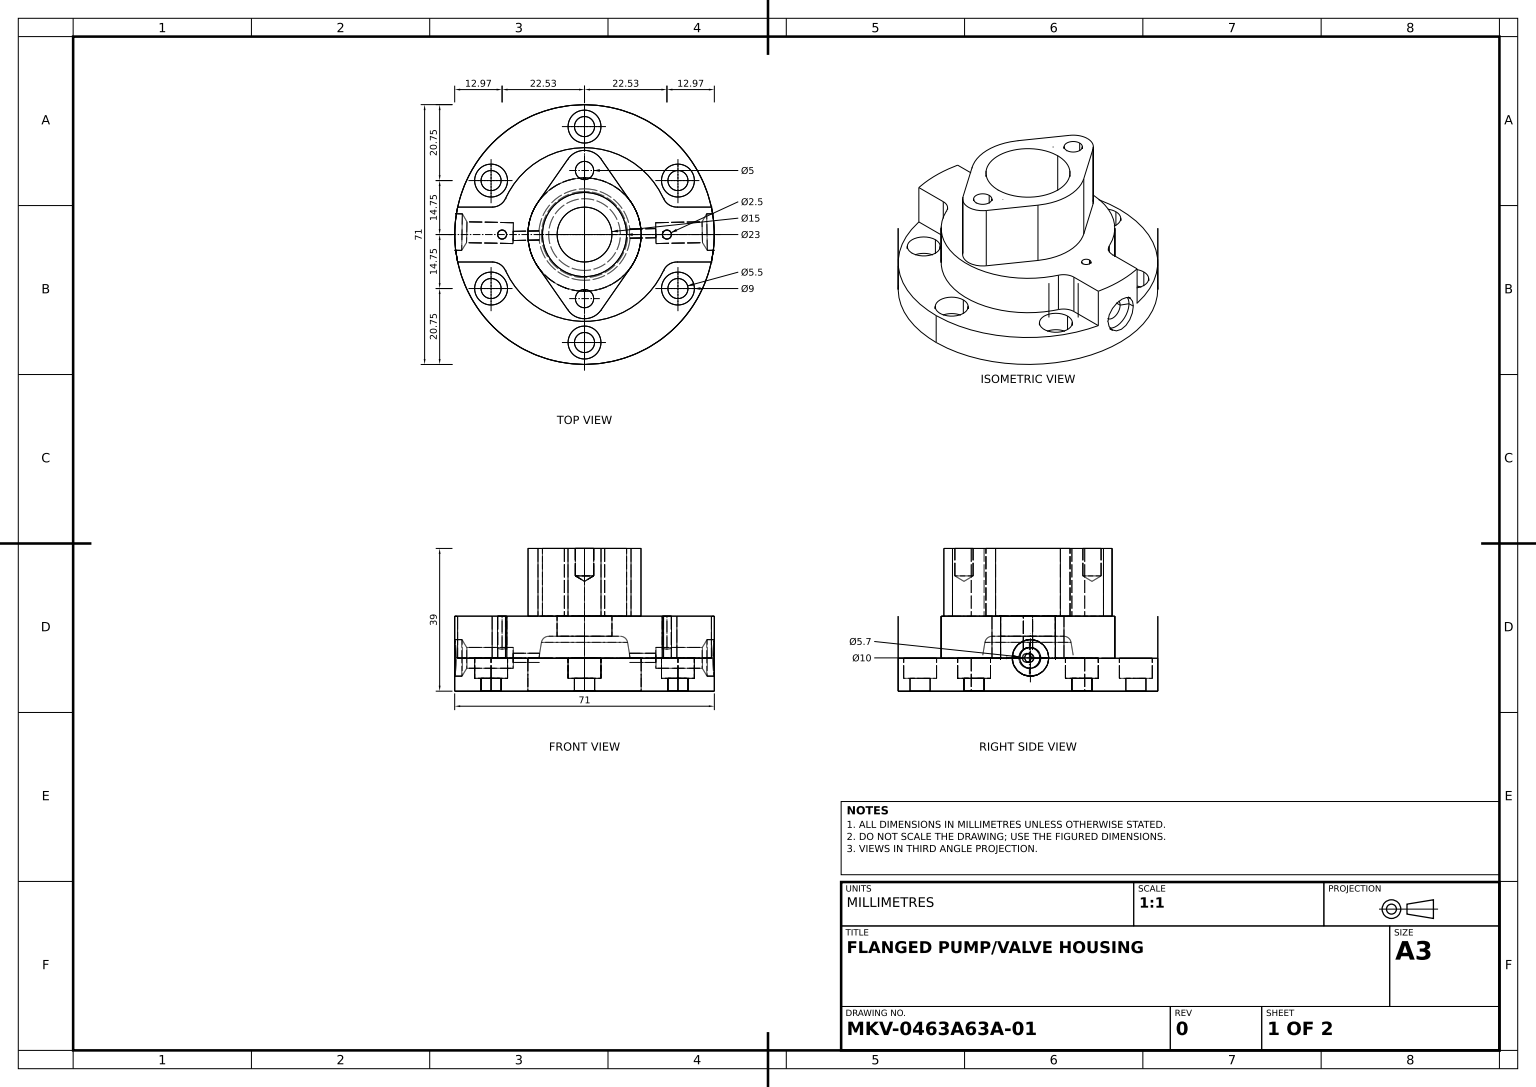
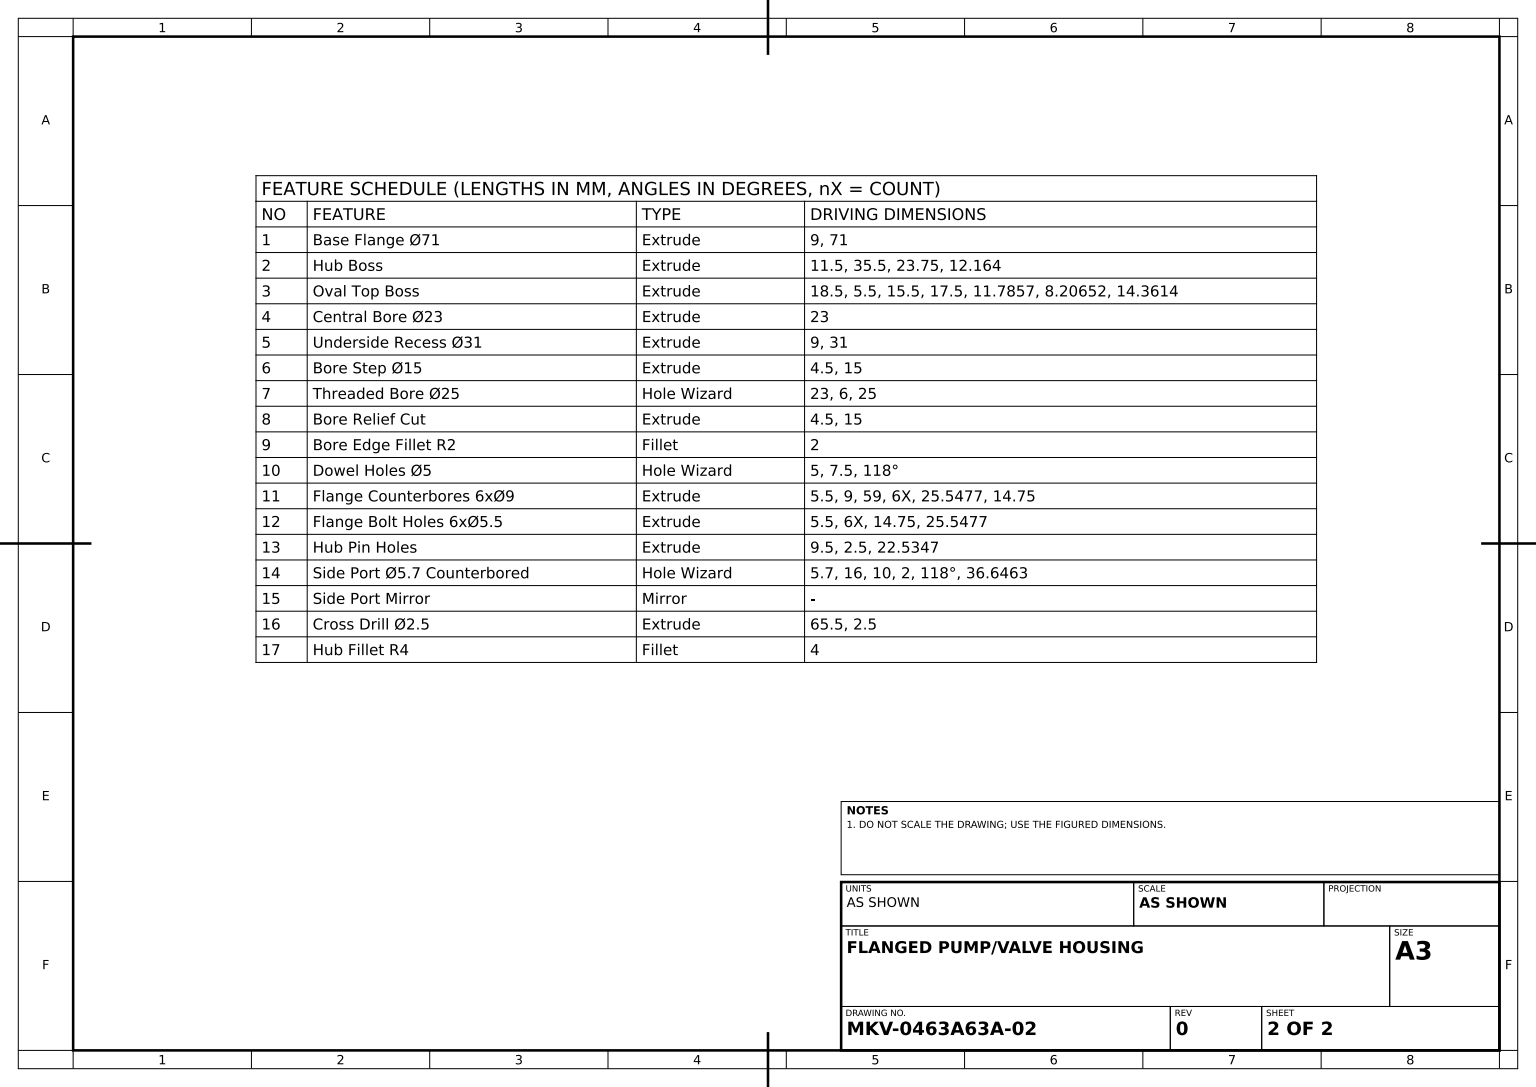
from build123d import *

# Parameters (mm, degrees)
BASE_FLANGE_SKETCH_R           = 35.5
BASE_FLANGE_71_DEPTH           = 9
HUB_BOSS_DEPTH                 = 11.5
OVAL_TOP_BOSS_DEPTH            = 18.5
CENTRAL_BORE_SKETCH_R          = 11.5
CENTRAL_BORE_23_DEPTH          = 18.5
UNDERSIDE_RECESS_SKETCH_R      = 15.5
UNDERSIDE_RECESS_31_DEPTH      = 9
BORE_STEP_SKETCH_R             = 7.5
BORE_STEP_15_DEPTH             = 4.5
BORE_RELIEF_SKETCH_R           = 7.5
BORE_RELIEF_CUT_DEPTH          = 4.5
BORE_EDGE_FILLET_R2_R          = 2
DOWEL_HOLES_5_D                = 5
DOWEL_HOLES_5_DEPTH            = 7.5
DOWEL_HOLES_5_TIP              = 1.502151548
FLANGE_COUNTERBORE_SKETCH_R    = 4.5
FLANGE_COUNTERBORES_6X_9_DEPTH = 5.5
FLANGE_BOLT_HOLE_SKETCH_R      = 2.75
FLANGE_BOLT_HOLES_6X_5_5_DEPTH = 5.5
HUB_PIN_HOLES_SKETCH_R         = 1.25
HUB_PIN_HOLES_DEPTH            = 9.5
CROSS_DRILL_SKETCH_R           = 1.25
CROSS_DRILL_2_5_DEPTH          = 65.5
HUB_FILLET_R4_R                = 4


with BuildPart() as part:
    # Base Flange Sketch → Base Flange _71 (new body)
    with BuildSketch(Plane(origin=(0, 0, 0), x_dir=(1, 0, 0), z_dir=(0, 1, 0))):
        with Locations(Location((0, 0, 0), (0, 0, 270))):
            Circle(BASE_FLANGE_SKETCH_R)
    extrude(amount=BASE_FLANGE_71_DEPTH)

    # Hub Profile Sketch → Hub Boss (add)
    with BuildSketch(Plane(origin=(0, 9, 0), x_dir=(1, 0, 0), z_dir=(0, 1, 0))):
        with BuildLine():
            Line((-22.534695472, 7.5), (-34.698703146, 7.5))
            ThreePointArc((-34.698703146, 7.5), (-35.5, 0), (-34.698703146, -7.5))
            Line((-34.698703146, -7.5), (-22.534695472, -7.5))
            ThreePointArc((-22.534695472, -7.5), (0, -23.75), (22.534695472, -7.5))
            Line((22.534695472, -7.5), (34.698703146, -7.5))
            ThreePointArc((34.698703146, -7.5), (35.5, 0), (34.698703146, 7.5))
            Line((34.698703146, 7.5), (22.534695472, 7.5))
            ThreePointArc((22.534695472, 7.5), (0, 23.75), (-22.534695472, 7.5))
        make_face()
    extrude(amount=HUB_BOSS_DEPTH)

    # Oval Top Boss Sketch → Oval Top Boss (add)
    with BuildSketch(Plane(origin=(0, 20.5, 0), x_dir=(1, 0, 0), z_dir=(0, 1, 0))):
        with BuildLine():
            Line((-4.513584937, 20.642857143), (-12.720103003, 8.857142857))
            ThreePointArc((-12.720103003, 8.857142857), (-15.5, 0), (-12.720103003, -8.857142857))
            Line((-12.720103003, -8.857142857), (-4.513584937, -20.642857143))
            ThreePointArc((-4.513584937, -20.642857143), (0, -23), (4.513584937, -20.642857143))
            Line((4.513584937, -20.642857143), (12.720103003, -8.857142857))
            ThreePointArc((12.720103003, -8.857142857), (15.5, 0), (12.720103003, 8.857142857))
            Line((12.720103003, 8.857142857), (4.513584937, 20.642857143))
            ThreePointArc((4.513584937, 20.642857143), (0, 23), (-4.513584937, 20.642857143))
        make_face()
    extrude(amount=OVAL_TOP_BOSS_DEPTH)

    # Central Bore Sketch → Central Bore _23 (cut)
    with BuildSketch(Plane(origin=(0, 39, 0), x_dir=(1, 0, 0), z_dir=(0, 1, 0))):
        with Locations(Location((0, 0, 0), (0, 0, 270))):
            Circle(CENTRAL_BORE_SKETCH_R)
    extrude(amount=-CENTRAL_BORE_23_DEPTH, mode=Mode.SUBTRACT)

    # Underside Recess Sketch → Underside Recess _31 (cut)
    with BuildSketch(Plane.XZ):
        with Locations(Location((0, 0, 0), (0, 0, 270))):
            Circle(UNDERSIDE_RECESS_SKETCH_R)
    extrude(amount=-UNDERSIDE_RECESS_31_DEPTH, mode=Mode.SUBTRACT)

    # Bore Step Sketch → Bore Step _15 (cut)
    with BuildSketch(Plane(origin=(0, 20.5, 0), x_dir=(1, 0, 0), z_dir=(0, 1, 0))):
        with Locations(Location((0, 0, 0), (0, 0, 270))):
            Circle(BORE_STEP_SKETCH_R)
    extrude(amount=-BORE_STEP_15_DEPTH, mode=Mode.SUBTRACT)

    # Sketch11 → Threaded Bore _25 (revolve, cut)
    with BuildSketch(Plane(origin=(0, 9, 0), x_dir=(0, 0, -1), z_dir=(1, 0, 0))):
        Polygon((0, 0), (0, 6), (11.5, 6), (12.5, 0), align=None)
    revolve(axis=Axis((0, 119, 0), (0, -1, 0)), mode=Mode.SUBTRACT)

    # Bore Relief Sketch → Bore Relief Cut (cut)
    with BuildSketch(Plane(origin=(0, 16, 0), x_dir=(1, 0, 0), z_dir=(0, 1, 0))):
        with Locations(Location((0, 0, 0), (0, 0, 270))):
            Circle(BORE_RELIEF_SKETCH_R)
    extrude(amount=-BORE_RELIEF_CUT_DEPTH, mode=Mode.SUBTRACT)

    # Bore Edge Fillet R2
    bore_edge_fillet_r2_edges = [part.edges().sort_by_distance(p)[0] for p in [
        (0, 15, 11.5),
    ]]
    fillet(bore_edge_fillet_r2_edges, radius=BORE_EDGE_FILLET_R2_R)

    # Dowel Holes _5
    with Locations(Plane(origin=(0, 39, 0), x_dir=(1, 0, 0), z_dir=(0, 1, 0))):
        with Locations((0, 17.5), (0, -17.5)):
            Hole(DOWEL_HOLES_5_D / 2, depth=DOWEL_HOLES_5_DEPTH)
            with Locations((0, 0, -(DOWEL_HOLES_5_DEPTH + DOWEL_HOLES_5_TIP / 2))):  # 118° drill point
                Cone(0, DOWEL_HOLES_5_D / 2, DOWEL_HOLES_5_TIP, mode=Mode.SUBTRACT)

    # Flange Counterbore Sketch → Flange Counterbores 6x_9 (cut)
    with BuildSketch(Plane(origin=(0, 9, 0), x_dir=(1, 0, 0), z_dir=(0, 1, 0))):
        with Locations(Location((0, 29.5, 0), (0, 0, 270))):
            Circle(FLANGE_COUNTERBORE_SKETCH_R)
        with Locations(Location((25.547749412, 14.75, 0), (0, 0, 270))):
            Circle(FLANGE_COUNTERBORE_SKETCH_R)
        with Locations(Location((25.547749412, -14.75, 0), (0, 0, 270))):
            Circle(FLANGE_COUNTERBORE_SKETCH_R)
        with Locations(Location((0, -29.5, 0), (0, 0, 270))):
            Circle(FLANGE_COUNTERBORE_SKETCH_R)
        with Locations(Location((-25.547749412, -14.75, 0), (0, 0, 270))):
            Circle(FLANGE_COUNTERBORE_SKETCH_R)
        with Locations(Location((-25.547749412, 14.75, 0), (0, 0, 270))):
            Circle(FLANGE_COUNTERBORE_SKETCH_R)
    extrude(amount=-FLANGE_COUNTERBORES_6X_9_DEPTH, mode=Mode.SUBTRACT)

    # Flange Bolt Hole Sketch → Flange Bolt Holes 6x_5.5 (cut)
    with BuildSketch(Plane(origin=(0, 3.5, 0), x_dir=(1, 0, 0), z_dir=(0, 1, 0))):
        with Locations(Location((0, 29.5, 0), (0, 0, 270))):
            Circle(FLANGE_BOLT_HOLE_SKETCH_R)
        with Locations(Location((25.547749412, 14.75, 0), (0, 0, 270))):
            Circle(FLANGE_BOLT_HOLE_SKETCH_R)
        with Locations(Location((25.547749412, -14.75, 0), (0, 0, 270))):
            Circle(FLANGE_BOLT_HOLE_SKETCH_R)
        with Locations(Location((0, -29.5, 0), (0, 0, 270))):
            Circle(FLANGE_BOLT_HOLE_SKETCH_R)
        with Locations(Location((-25.547749412, -14.75, 0), (0, 0, 270))):
            Circle(FLANGE_BOLT_HOLE_SKETCH_R)
        with Locations(Location((-25.547749412, 14.75, 0), (0, 0, 270))):
            Circle(FLANGE_BOLT_HOLE_SKETCH_R)
    extrude(amount=-FLANGE_BOLT_HOLES_6X_5_5_DEPTH, mode=Mode.SUBTRACT)

    # Hub Pin Holes Sketch → Hub Pin Holes (cut)
    with BuildSketch(Plane(origin=(0, 20.5, 0), x_dir=(1, 0, 0), z_dir=(0, 1, 0))):
        with Locations(Location((-22.534695472, 0, 0), (0, 0, 270))):
            Circle(HUB_PIN_HOLES_SKETCH_R)
        with Locations(Location((22.534695472, 0, 0), (0, 0, 90))):
            Circle(HUB_PIN_HOLES_SKETCH_R)
    extrude(amount=-HUB_PIN_HOLES_DEPTH, mode=Mode.SUBTRACT)

    # Sketch22 → Side Port _5.7 Counterbored (revolve, cut)
    with BuildSketch(Plane(origin=(-35.493017285, 9.093847626, -0.704076681), x_dir=(-0.0198331459501574, 0, 0.9998033038161656), z_dir=(0, 1, 0))):
        Polygon((0, 0), (0, 16), (2.85, 16), (2.85, 3.291850331), (5, 2), (5, 0), align=None)
    side_port_5_7_counterbored = revolve(axis=Axis((-41.621835432, 9.093847626, -0.82565434), (0.9998033038161656, 0, 0.019833145950157397)), mode=Mode.SUBTRACT)

    # Side Port Mirror: Side Port _5.7 Counterbored across plane
    add(side_port_5_7_counterbored.mirror(Plane(origin=(0, 0, 0), x_dir=(0, 0, 1), z_dir=(1, 0, 0))), mode=Mode.SUBTRACT)

    # Cross Drill Sketch → Cross Drill _2.5 (cut)
    with BuildSketch(Plane(origin=(19.496164424, 0, -0.386746346), x_dir=(-0.019833145950157404, 0, -0.9998033038161656), z_dir=(0.9998033038161657, 0, -0.019833145950157404))):
        with Locations((0, 9.093847626)):
            Circle(CROSS_DRILL_SKETCH_R)
    extrude(amount=-CROSS_DRILL_2_5_DEPTH, mode=Mode.SUBTRACT)

    # Hub Fillet R4
    hub_fillet_r4_edges = [part.edges().sort_by_distance(p)[0] for p in [
        (-22.534695472, 14.75, 7.5),
        (22.534695472, 14.75, 7.5),
        (22.534695472, 14.75, -7.5),
        (-22.534695472, 14.75, -7.5),
    ]]
    fillet(hub_fillet_r4_edges, radius=HUB_FILLET_R4_R)


solid = part.part
